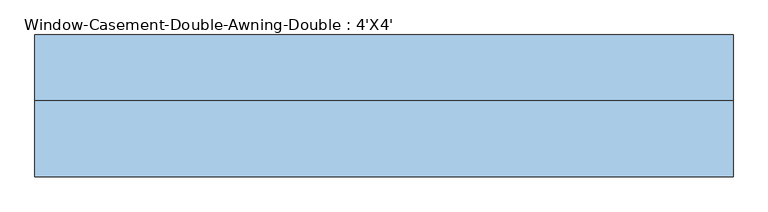
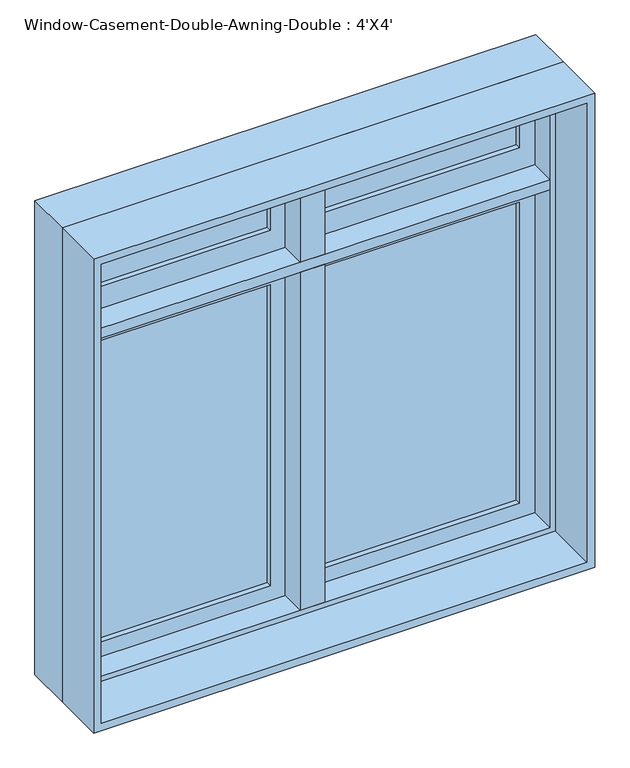
"""IFC4 building model written with IfcOpenShell, lengths in millimetres: window geometry, Window-Casement-Double-Awning-Double : 4'X4'."""

from ifc_helpers import new_model, si_unit, frame, origin, place, context, project, spatial, polyline, outline, extrude, faceted_brep, source, transform, mapped, element, save


def window_casement_double_awning_double_4_x4_dd9041c6(model_context):
    return source(origin(), model_context, "Body", "SolidModel", [
        faceted_brep([(577.85, 82.55, 2101.85), (577.85, 19.05, 2101.85), (-577.85, 19.05, 2101.85), (-577.85, 82.55, 2101.85), (596.9, 133.35, 2120.9), (596.9, 82.55, 2120.9), (-596.9, 82.55, 2120.9), (-596.9, 133.35, 2120.9), (609.6, 19.05, 2133.6), (609.6, 133.35, 2133.6), (-609.6, 133.35, 2133.6), (-609.6, 19.05, 2133.6), (-577.85, 19.05, 946.15), (-577.85, 82.55, 946.15), (-596.9, 82.55, 927.1), (-596.9, 133.35, 927.1), (-609.6, 133.35, 914.4), (-609.6, 19.05, 914.4), (577.85, 19.05, 946.15), (577.85, 82.55, 946.15), (596.9, 82.55, 927.1), (596.9, 133.35, 927.1), (609.6, 133.35, 914.4), (609.6, 19.05, 914.4)], [[[0, 1, 2, 3]], [[4, 5, 6, 7]], [[8, 9, 10, 11]], [[3, 2, 12, 13]], [[7, 6, 14, 15]], [[11, 10, 16, 17]], [[13, 12, 18, 19]], [[15, 14, 20, 21]], [[17, 16, 22, 23]], [[11, 17, 23, 8], [1, 18, 12, 2]], [[19, 18, 1, 0]], [[5, 20, 14, 6], [3, 13, 19, 0]], [[21, 20, 5, 4]], [[23, 22, 9, 8]], [[9, 22, 16, 10], [7, 15, 21, 4]]]),
        extrude(outline(polyline([(2133.6, -609.6), (914.4, -609.6), (914.4, 609.6), (2133.6, 609.6), (2133.6, -609.6)]), holes=[polyline([(2114.55, 590.55), (933.45, 590.55), (933.45, -590.55), (2114.55, -590.55), (2114.55, 590.55)])]), frame((0.0, -114.3, 0.0), z_axis=(0.0, 1.0, 0.0), x_axis=(0.0, 0.0, 1.0)), (0.0, 0.0, 1.0), 133.35),
        extrude(outline(polyline([(927.1, 596.9), (1816.1, 596.9), (1816.1, 9.525), (927.1, 9.525), (927.1, 596.9)]), holes=[polyline([(984.25, 66.675), (1758.95, 66.675), (1758.95, 539.75), (984.25, 539.75), (984.25, 66.675)])]), frame((0.0, 82.55, 0.0), z_axis=(0.0, 1.0, 0.0), x_axis=(0.0, 0.0, 1.0)), (0.0, 0.0, 1.0), 44.45),
        extrude(outline(polyline([(1816.1, -596.9), (927.1, -596.9), (927.1, -9.525), (1816.1, -9.525), (1816.1, -596.9)]), holes=[polyline([(1758.95, -66.675), (984.25, -66.675), (984.25, -539.75), (1758.95, -539.75), (1758.95, -66.675)])]), frame((0.0, 82.55, 0.0), z_axis=(0.0, 1.0, 0.0), x_axis=(0.0, 0.0, 1.0)), (0.0, 0.0, 1.0), 44.45),
        extrude(outline(polyline([(539.75, 114.3), (539.75, 107.95), (66.675, 107.95), (66.675, 114.3), (539.75, 114.3)])), frame((0.0, 0.0, 984.25), z_axis=(0.0, 0.0, 1.0), x_axis=(1.0, 0.0, 0.0)), (0.0, 0.0, 1.0), 774.7),
        extrude(outline(polyline([(66.675, 95.25), (66.675, 101.6), (539.75, 101.6), (539.75, 95.25), (66.675, 95.25)])), frame((0.0, 0.0, 984.25), z_axis=(0.0, 0.0, 1.0), x_axis=(1.0, 0.0, 0.0)), (0.0, 0.0, 1.0), 774.7),
        extrude(outline(polyline([(-66.675, 114.3), (-66.675, 107.95), (-539.75, 107.95), (-539.75, 114.3), (-66.675, 114.3)])), frame((0.0, 0.0, 984.25), z_axis=(0.0, 0.0, 1.0), x_axis=(1.0, 0.0, 0.0)), (0.0, 0.0, 1.0), 774.7),
        extrude(outline(polyline([(-539.75, 95.25), (-539.75, 101.6), (-66.675, 101.6), (-66.675, 95.25), (-539.75, 95.25)])), frame((0.0, 0.0, 984.25), z_axis=(0.0, 0.0, 1.0), x_axis=(1.0, 0.0, 0.0)), (0.0, 0.0, 1.0), 774.7),
        faceted_brep([(9.525, 133.35, 1816.1), (-9.525, 133.35, 1816.1), (-9.525, 82.55, 1816.1), (-30.1625, 82.55, 1816.1), (-30.1625, 19.05, 1816.1), (30.1625, 19.05, 1816.1), (30.1625, 82.55, 1816.1), (9.525, 82.55, 1816.1), (9.525, 133.35, 927.1), (9.525, 82.55, 927.1), (-9.525, 82.55, 927.1), (-9.525, 133.35, 927.1), (-9.525, 82.55, 946.15), (-30.1625, 82.55, 946.15), (-30.1625, 19.05, 946.15), (30.1625, 19.05, 946.15), (30.1625, 82.55, 946.15), (9.525, 82.55, 946.15)], [[[0, 1, 2, 3, 4, 5, 6, 7]], [[8, 9, 10, 11]], [[1, 0, 8, 11]], [[2, 1, 11, 10, 12]], [[3, 2, 12, 13]], [[4, 3, 13, 14]], [[5, 4, 14, 15]], [[6, 5, 15, 16]], [[7, 6, 16, 17]], [[0, 7, 17, 9, 8]], [[17, 12, 10, 9]], [[12, 17, 16, 15, 14, 13]]]),
        extrude(outline(polyline([(-66.675, 114.3), (-66.675, 107.95), (-539.75, 107.95), (-539.75, 114.3), (-66.675, 114.3)])), frame((0.0, 0.0, 1898.65), z_axis=(0.0, 0.0, 1.0), x_axis=(1.0, 0.0, 0.0)), (0.0, 0.0, 1.0), 165.1),
        extrude(outline(polyline([(-539.75, 95.25), (-539.75, 101.6), (-66.675, 101.6), (-66.675, 95.25), (-539.75, 95.25)])), frame((0.0, 0.0, 1898.65), z_axis=(0.0, 0.0, 1.0), x_axis=(1.0, 0.0, 0.0)), (0.0, 0.0, 1.0), 165.1),
        extrude(outline(polyline([(596.9, 133.35), (596.9, 82.55), (577.85, 82.55), (577.85, 19.05), (-577.85, 19.05), (-577.85, 82.55), (-596.9, 82.55), (-596.9, 133.35), (596.9, 133.35)])), frame((0.0, 0.0, 1816.1), z_axis=(0.0, 0.0, 1.0), x_axis=(1.0, 0.0, 0.0)), (0.0, 0.0, 1.0), 25.4),
        faceted_brep([(9.525, 82.55, 2120.9), (9.525, 133.35, 2120.9), (-9.525, 133.35, 2120.9), (-9.525, 82.55, 2120.9), (-9.525, 82.55, 1841.5), (-9.525, 133.35, 1841.5), (9.525, 133.35, 1841.5), (9.525, 82.55, 1841.5), (30.1625, 82.55, 1841.5), (30.1625, 19.05, 1841.5), (-30.1625, 19.05, 1841.5), (-30.1625, 82.55, 1841.5), (-30.1625, 82.55, 2101.85), (-9.525, 82.55, 2101.85), (-30.1625, 19.05, 2101.85), (30.1625, 19.05, 2101.85), (30.1625, 82.55, 2101.85), (9.525, 82.55, 2101.85)], [[[0, 1, 2, 3]], [[4, 5, 6, 7, 8, 9, 10, 11]], [[4, 11, 12, 13]], [[11, 10, 14, 12]], [[10, 9, 15, 14]], [[9, 8, 16, 15]], [[8, 7, 17, 16]], [[1, 0, 17, 7, 6]], [[2, 1, 6, 5]], [[3, 2, 5, 4, 13]], [[17, 13, 12, 14, 15, 16]], [[13, 17, 0, 3]]]),
        extrude(outline(polyline([(2120.9, 9.525), (1841.5, 9.525), (1841.5, 596.9), (2120.9, 596.9), (2120.9, 9.525)]), holes=[polyline([(2063.75, 539.75), (1898.65, 539.75), (1898.65, 66.675), (2063.75, 66.675), (2063.75, 539.75)])]), frame((0.0, 82.55, 0.0), z_axis=(0.0, 1.0, 0.0), x_axis=(0.0, 0.0, 1.0)), (0.0, 0.0, 1.0), 44.45),
        extrude(outline(polyline([(1841.5, -9.525), (2120.9, -9.525), (2120.9, -596.9), (1841.5, -596.9), (1841.5, -9.525)]), holes=[polyline([(1898.65, -539.75), (2063.75, -539.75), (2063.75, -66.675), (1898.65, -66.675), (1898.65, -539.75)])]), frame((0.0, 82.55, 0.0), z_axis=(0.0, 1.0, 0.0), x_axis=(0.0, 0.0, 1.0)), (0.0, 0.0, 1.0), 44.45),
        extrude(outline(polyline([(66.675, 114.3), (539.75, 114.3), (539.75, 107.95), (66.675, 107.95), (66.675, 114.3)])), frame((0.0, 0.0, 1898.65), z_axis=(0.0, 0.0, 1.0), x_axis=(1.0, 0.0, 0.0)), (0.0, 0.0, 1.0), 165.1),
        extrude(outline(polyline([(539.75, 95.25), (66.675, 95.25), (66.675, 101.6), (539.75, 101.6), (539.75, 95.25)])), frame((0.0, 0.0, 1898.65), z_axis=(0.0, 0.0, 1.0), x_axis=(1.0, 0.0, 0.0)), (0.0, 0.0, 1.0), 165.1),
    ])


if __name__ == "__main__":
    model = new_model("IFC4")
    model_context = context("Model", 3, world=origin())
    ifc_project = project(units=[si_unit("LENGTHUNIT", "METRE", prefix="MILLI")], contexts=[model_context])
    site = spatial("IfcSite", under=ifc_project)
    building = spatial("IfcBuilding", under=site)
    placement = place(None, origin())
    window_casement_double_awning_double_4_x4_shape = window_casement_double_awning_double_4_x4_dd9041c6(model_context)
    element("IfcWindow", 1, ObjectType="Window-Casement-Double-Awning-Double : 4'X4'", at=placement, inside=building, context=model_context, shape_type="MappedRepresentation", body=[
        mapped(window_casement_double_awning_double_4_x4_shape, transform((0.0, 0.0, 0.0), x_axis=(1.0, 0.0, 0.0), y_axis=(0.0, 1.0, 0.0), z_axis=(0.0, 0.0, 1.0))),
    ])
    save(model, "model.ifc")

# Revit data of these elements
# Type "Window-Casement-Double-Awning-Double : 4'X4'"
#   Type Mark = "19"
#   Fire Rating = "0.5h"
#   Assembly Code = "B2020100"
#   Analytic Construction = "Double glazing - domestic"
#   Window Inset [instance default] = 0' - 0"
#   Wall Thickness [instance default] = 0' - 6"
#   Interior Wall Closure [instance default] = 0' - 2 1/4"
#   Half Width = 2' - 0"
#   Visual Light Transmittance = 0.81
#   Transom Height = 1' - 0"
#   Thermal Resistance (R) = 1.8146 (h·ft²·°F)/BTU
#   Solar Heat Gain Coefficient = 0.76
#   Rough Width = 4' - 0 1/2"
#   Rough Height = 4' - 0 1/2"
#   Open Window Height = 3' - 0"
#   Frame Extension [instance default] = 0' - 0 1/4"
#   Height = 4' - 0"
#   Heat Transfer Coefficient (U) = 0.5511 BTU/(h·ft²·°F)
#   Exterior Wall Closure [instance default] = 0' - 1 1/4"
#   Extension Jamb [instance default] = 0' - 2 1/4"
#   Default Sill Height = 3' - 0"
#   Width = 4' - 0"
#   Top Muntin Visibility = yes
#   Bottom Muntin Visibility = yes
#   Interior Trim Visibility [instance default] = yes
#   Exterior Trim Visibility [instance default] = yes
#   Extension Jamb Visibility [instance default] = yes
#   Interior Trim Material = Wood - Stained
#   Muntin Pattern = Muntin Pattern_2x2 : Muntin Pattern_2x2
#   Interior Trim = Trim-Window-Interior-Flat : Picture Frame
#   Interior Frame Material = Wood - Stained
#   Glass Panel Material = Glass
#   Exterior Trim Material = Clad - White
#   Exterior Trim = Trim-Window-Exterior-Flat : with Sill
#   Exterior Frame Material = Clad - White
#   Wall Closure = (empty or 0)
# Element 1 (IfcWindow, "Window-Casement-Double-Awning-Double : 4'X4'")
#   Wall Thickness = 0' - 9"
#   Extension Jamb = 0' - 5 1/4"
#   Materials on its faces: "Wood - Stained", "Glass", "Clad - White"
# Materials
#   "Wood - Stained": class "Wood", colour RGB 224 178 126, transparency 0, Cost = 0
#   "Glass": class "Glass", colour RGB 0 128 192, transparency 0.75, Description = "Soda Lime Glass", Cost = 0
#   "Clad - White": class "Wood", colour RGB 242 242 238, transparency 0, Cost = 0
